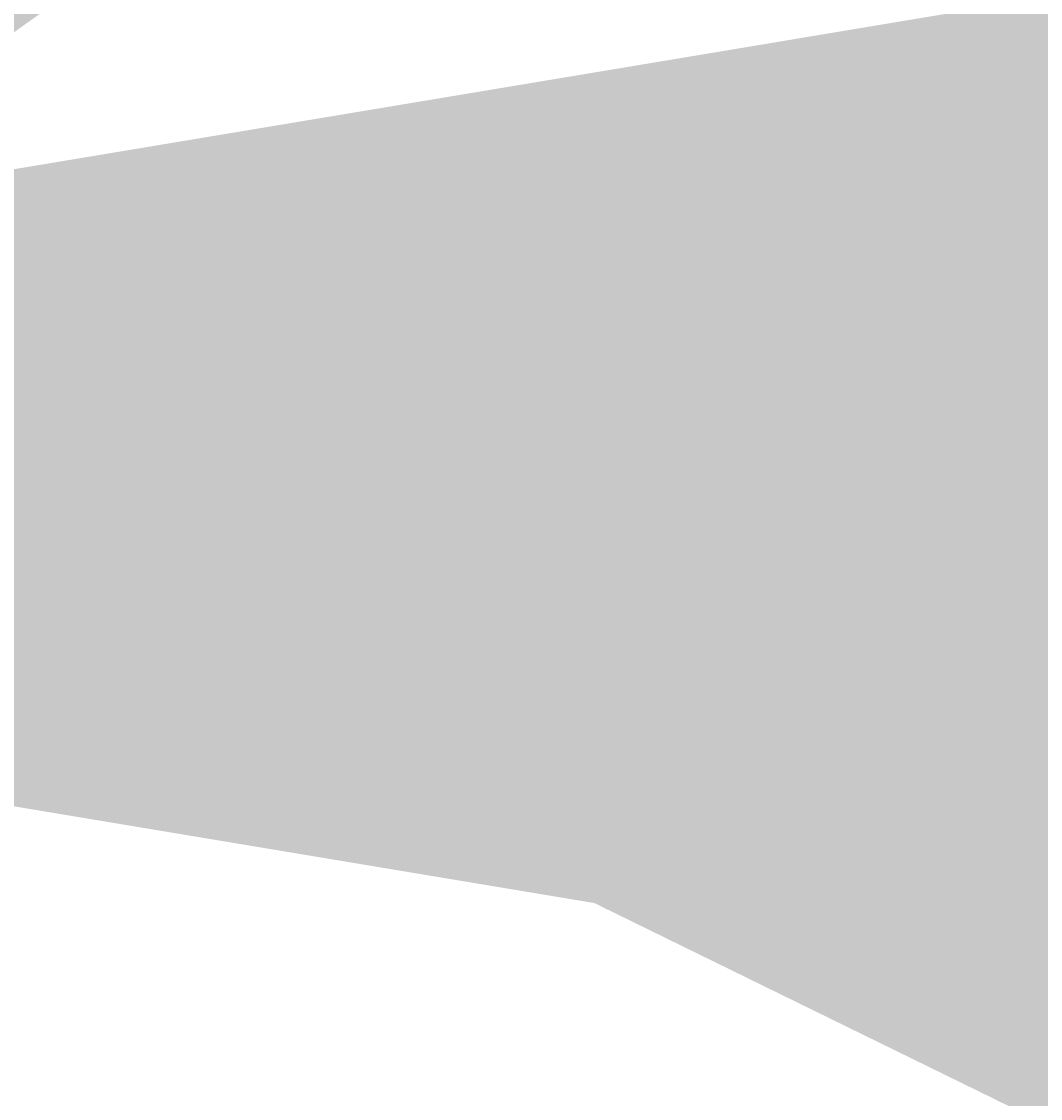
# Model space of a CAD drawing. Units: millimetres. Extents: x -22994 to 29398, y -19990 to 20176.
# Tile 127 of 135: x 480 to 1004, y -212 to 341. Entities that reach past the tile are written whole.
import ezdxf

# ---------------------------------------------------------------- set-up
doc = ezdxf.new("R2010")
doc.units = ezdxf.units.MM
doc.header["$MEASUREMENT"] = 0
doc.layers.add('M-DIMS', color=2, linetype='Continuous', lineweight=18)
doc.styles.get("Standard").update_dxf_attribs({"font": 'arial.ttf'})
doc.dimstyles.get("Standard").update_dxf_attribs({"dimtxt": 0.18, "dimasz": 10000, "dimexe": 0.18, "dimexo": 0.0625, "dimgap": 0.09, "dimtad": 0, "dimtih": 1, "dimtoh": 1, "dimdec": 0, "dimzin": 0, "dimdsep": 46, "dimtxsty": 'Standard', "dimcen": 0.09, "dimadec": 0, "dimazin": 0, "dimtfac": 1, "dimtdec": 0, "dimtofl": 0, "dimtmove": 0, "dimatfit": 3, "dimfxl": 1, "dimtolj": 1, "dimtzin": 0, "dimlwd": 30, "dimarcsym": 0})

# ---------------------------------------------------------------- blocks, each defined once
blk = doc.blocks.new('*D2')
at = {"layer": 'Defpoints', "color": 0, "transparency": 16777216}
for p in [(6.68, 10.27), (290.85, 10.27), (290.85, -5.08)]:
    blk.add_point(p, dxfattribs=at)
at = {"layer": 'M-DIMS', "color": 0, "lineweight": -2, "transparency": 16777216}
for p, q in [((6.68, 10.21), (6.68, -5.26)), ((290.85, 10.21), (290.85, -5.26))]:
    blk.add_line(p, q, dxfattribs=at)
at = {"layer": 'M-DIMS', "color": 0, "lineweight": 30, "transparency": 16777216}
for p, q in [((-9993.32, -5.08), (-19993.32, -5.08)), ((10290.85, -5.08), (20290.85, -5.08))]:
    blk.add_line(p, q, dxfattribs=at)
at = {"layer": 'M-DIMS', "color": 0, "transparency": 16777216}
for points in [[(-9993.32, 1661.59), (-9993.32, -1671.75), (6.68, -5.08)], [(10290.85, 1661.59), (10290.85, -1671.75), (290.85, -5.08)]]:
    blk.add_solid(points, dxfattribs=at)
at = {"layer": 'M-DIMS', "color": 0, "transparency": 16777216, "insert": (148.76, -5.08), "char_height": 0.18, "attachment_point": 5}
blk.add_mtext('\\A1;284.2', dxfattribs=at)
blk = doc.blocks.new('*D3')
at = {"layer": 'Defpoints', "color": 0, "transparency": 16777216}
for p in [(110.26, 204.17), (110.26, 176.37), (95.83, 127.97)]:
    blk.add_point(p, dxfattribs=at)
at = {"layer": 'M-DIMS', "color": 0, "lineweight": 30, "transparency": 16777216}
for p, q in [((-9904.17, 204.17), (-19904.17, 204.17)), ((10110.26, 204.17), (20110.26, 204.17))]:
    blk.add_line(p, q, dxfattribs=at)
at = {"layer": 'M-DIMS', "color": 0, "lineweight": -2, "transparency": 16777216}
for p, q in [((95.83, 128.03), (95.83, 204.35)), ((110.26, 176.43), (110.26, 204.35))]:
    blk.add_line(p, q, dxfattribs=at)
at = {"layer": 'M-DIMS', "color": 0, "transparency": 16777216}
for points in [[(-9904.17, 1870.83), (-9904.17, -1462.5), (95.83, 204.17)], [(10110.26, 1870.83), (10110.26, -1462.5), (110.26, 204.17)]]:
    blk.add_solid(points, dxfattribs=at)
at = {"layer": 'M-DIMS', "color": 0, "transparency": 16777216, "insert": (103.05, 204.17), "char_height": 0.18, "attachment_point": 5}
blk.add_mtext('\\A1;14.432', dxfattribs=at)
blk = doc.blocks.new('*D4')
at = {"layer": 'Defpoints', "color": 0, "transparency": 16777216}
for p in [(116.26, 204.17), (110.26, 176.37), (116.26, 176.37)]:
    blk.add_point(p, dxfattribs=at)
at = {"layer": 'M-DIMS', "color": 0, "lineweight": 30, "transparency": 16777216}
for p, q in [((-9889.74, 204.17), (-19889.74, 204.17)), ((10116.26, 204.17), (20116.26, 204.17))]:
    blk.add_line(p, q, dxfattribs=at)
at = {"layer": 'M-DIMS', "color": 0, "lineweight": -2, "transparency": 16777216}
for p, q in [((110.26, 176.43), (110.26, 204.35)), ((116.26, 176.43), (116.26, 204.35))]:
    blk.add_line(p, q, dxfattribs=at)
at = {"layer": 'M-DIMS', "color": 0, "transparency": 16777216}
for points in [[(-9889.74, 1870.83), (-9889.74, -1462.5), (110.26, 204.17)], [(10116.26, 1870.83), (10116.26, -1462.5), (116.26, 204.17)]]:
    blk.add_solid(points, dxfattribs=at)
at = {"layer": 'M-DIMS', "color": 0, "transparency": 16777216, "insert": (113.26, 204.17), "char_height": 0.18, "attachment_point": 5}
blk.add_mtext('\\A1;6', dxfattribs=at)
blk = doc.blocks.new('*D5')
at = {"layer": 'Defpoints', "color": 0, "transparency": 16777216}
for p in [(181.26, 204.17), (116.26, 176.37), (181.26, 176.37)]:
    blk.add_point(p, dxfattribs=at)
at = {"layer": 'M-DIMS', "color": 0, "lineweight": 30, "transparency": 16777216}
for p, q in [((-9883.74, 204.17), (-19883.74, 204.17)), ((10181.26, 204.17), (20181.26, 204.17))]:
    blk.add_line(p, q, dxfattribs=at)
at = {"layer": 'M-DIMS', "color": 0, "lineweight": -2, "transparency": 16777216}
for p, q in [((116.26, 176.43), (116.26, 204.35)), ((181.26, 176.43), (181.26, 204.35))]:
    blk.add_line(p, q, dxfattribs=at)
at = {"layer": 'M-DIMS', "color": 0, "transparency": 16777216}
for points in [[(-9883.74, 1870.83), (-9883.74, -1462.5), (116.26, 204.17)], [(10181.26, 1870.83), (10181.26, -1462.5), (181.26, 204.17)]]:
    blk.add_solid(points, dxfattribs=at)
at = {"layer": 'M-DIMS', "color": 0, "transparency": 16777216, "insert": (148.76, 204.17), "char_height": 0.18, "attachment_point": 5}
blk.add_mtext('\\A1;65', dxfattribs=at)
blk = doc.blocks.new('*D6')
at = {"layer": 'Defpoints', "color": 0, "transparency": 16777216}
for p in [(187.26, 204.17), (181.26, 176.37), (187.26, 176.37)]:
    blk.add_point(p, dxfattribs=at)
at = {"layer": 'M-DIMS', "color": 0, "lineweight": 30, "transparency": 16777216}
for p, q in [((-9818.74, 204.17), (-19818.74, 204.17)), ((10187.26, 204.17), (20187.26, 204.17))]:
    blk.add_line(p, q, dxfattribs=at)
at = {"layer": 'M-DIMS', "color": 0, "lineweight": -2, "transparency": 16777216}
for p, q in [((181.26, 176.43), (181.26, 204.35)), ((187.26, 176.43), (187.26, 204.35))]:
    blk.add_line(p, q, dxfattribs=at)
at = {"layer": 'M-DIMS', "color": 0, "transparency": 16777216}
for points in [[(-9818.74, 1870.83), (-9818.74, -1462.5), (181.26, 204.17)], [(10187.26, 1870.83), (10187.26, -1462.5), (187.26, 204.17)]]:
    blk.add_solid(points, dxfattribs=at)
at = {"layer": 'M-DIMS', "color": 0, "transparency": 16777216, "insert": (184.26, 204.17), "char_height": 0.18, "attachment_point": 5}
blk.add_mtext('\\A1;6', dxfattribs=at)
blk = doc.blocks.new('*D7')
at = {"layer": 'Defpoints', "color": 0, "transparency": 16777216}
for p in [(201.7, 204.17), (187.26, 176.37), (201.7, 127.97)]:
    blk.add_point(p, dxfattribs=at)
at = {"layer": 'M-DIMS', "color": 0, "lineweight": 30, "transparency": 16777216}
for p, q in [((-9812.74, 204.17), (-19812.74, 204.17)), ((10201.7, 204.17), (20201.7, 204.17))]:
    blk.add_line(p, q, dxfattribs=at)
at = {"layer": 'M-DIMS', "color": 0, "lineweight": -2, "transparency": 16777216}
for p, q in [((187.26, 176.43), (187.26, 204.35)), ((201.7, 128.03), (201.7, 204.35))]:
    blk.add_line(p, q, dxfattribs=at)
at = {"layer": 'M-DIMS', "color": 0, "transparency": 16777216}
for points in [[(-9812.74, 1870.83), (-9812.74, -1462.5), (187.26, 204.17)], [(10201.7, 1870.83), (10201.7, -1462.5), (201.7, 204.17)]]:
    blk.add_solid(points, dxfattribs=at)
at = {"layer": 'M-DIMS', "color": 0, "transparency": 16777216, "insert": (194.48, 204.17), "char_height": 0.18, "attachment_point": 5}
blk.add_mtext('\\A1;14.432', dxfattribs=at)
blk = doc.blocks.new('*D8')
at = {"layer": 'Defpoints', "color": 0, "transparency": 16777216}
for p in [(227.65, 204.17), (227.65, 146.73), (201.7, 127.97)]:
    blk.add_point(p, dxfattribs=at)
at = {"layer": 'M-DIMS', "color": 0, "lineweight": 30, "transparency": 16777216}
for p, q in [((-9798.3, 204.17), (-19798.3, 204.17)), ((10227.65, 204.17), (20227.65, 204.17))]:
    blk.add_line(p, q, dxfattribs=at)
at = {"layer": 'M-DIMS', "color": 0, "lineweight": -2, "transparency": 16777216}
for p, q in [((201.7, 128.03), (201.7, 204.35)), ((227.65, 146.79), (227.65, 204.35))]:
    blk.add_line(p, q, dxfattribs=at)
at = {"layer": 'M-DIMS', "color": 0, "transparency": 16777216}
for points in [[(-9798.3, 1870.83), (-9798.3, -1462.5), (201.7, 204.17)], [(10227.65, 1870.83), (10227.65, -1462.5), (227.65, 204.17)]]:
    blk.add_solid(points, dxfattribs=at)
at = {"layer": 'M-DIMS', "color": 0, "transparency": 16777216, "insert": (214.67, 204.17), "char_height": 0.18, "attachment_point": 5}
blk.add_mtext('\\A1;25.95', dxfattribs=at)
blk = doc.blocks.new('*D9')
at = {"layer": 'Defpoints', "color": 0, "transparency": 16777216}
for p in [(187.26, 176.37), (306.2, 176.37), (290.85, 10.27)]:
    blk.add_point(p, dxfattribs=at)
at = {"layer": 'M-DIMS', "color": 0, "lineweight": 30, "transparency": 16777216}
for p, q in [((306.2, 10176.37), (306.2, 20176.37)), ((306.2, -9989.73), (306.2, -19989.73))]:
    blk.add_line(p, q, dxfattribs=at)
at = {"layer": 'M-DIMS', "color": 0, "lineweight": -2, "transparency": 16777216}
for p, q in [((187.33, 176.37), (306.38, 176.37)), ((290.91, 10.27), (306.38, 10.27))]:
    blk.add_line(p, q, dxfattribs=at)
at = {"layer": 'M-DIMS', "color": 0, "transparency": 16777216}
for points in [[(-1360.46, 10176.37), (1972.87, 10176.37), (306.2, 176.37)], [(-1360.46, -9989.73), (1972.87, -9989.73), (306.2, 10.27)]]:
    blk.add_solid(points, dxfattribs=at)
at = {"layer": 'M-DIMS', "color": 0, "transparency": 16777216, "insert": (306.2, 93.32), "char_height": 0.18, "attachment_point": 5}
blk.add_mtext('\\A1;166.1', dxfattribs=at)
blk = doc.blocks.new('*D10')
at = {"layer": 'Defpoints', "color": 0, "transparency": 16777216}
for p in [(125.65, 136.07), (133.35, 136.07), (133.35, -5.08)]:
    blk.add_point(p, dxfattribs=at)
at = {"layer": 'M-DIMS', "color": 0, "lineweight": -2, "transparency": 16777216}
for p, q in [((125.65, 136.01), (125.65, -5.26)), ((133.35, 136.01), (133.35, -5.26))]:
    blk.add_line(p, q, dxfattribs=at)
at = {"layer": 'M-DIMS', "color": 0, "lineweight": 30, "transparency": 16777216}
for p, q in [((-9874.35, -5.08), (-19874.35, -5.08)), ((10133.35, -5.08), (20133.35, -5.08))]:
    blk.add_line(p, q, dxfattribs=at)
at = {"layer": 'M-DIMS', "color": 0, "transparency": 16777216}
for points in [[(-9874.35, 1661.59), (-9874.35, -1671.75), (125.65, -5.08)], [(10133.35, 1661.59), (10133.35, -1671.75), (133.35, -5.08)]]:
    blk.add_solid(points, dxfattribs=at)
at = {"layer": 'M-DIMS', "color": 0, "transparency": 16777216, "insert": (129.5, -5.08), "char_height": 0.18, "attachment_point": 5}
blk.add_mtext('\\A1;7.696', dxfattribs=at)
blk = doc.blocks.new('*D11')
at = {"layer": 'Defpoints', "color": 0, "transparency": 16777216}
for p in [(133.35, 136.07), (135.65, 136.07), (135.65, -5.08)]:
    blk.add_point(p, dxfattribs=at)
at = {"layer": 'M-DIMS', "color": 0, "lineweight": -2, "transparency": 16777216}
for p, q in [((133.35, 136.01), (133.35, -5.26)), ((135.65, 136.01), (135.65, -5.26))]:
    blk.add_line(p, q, dxfattribs=at)
at = {"layer": 'M-DIMS', "color": 0, "lineweight": 30, "transparency": 16777216}
for p, q in [((-9866.65, -5.08), (-19866.65, -5.08)), ((10135.65, -5.08), (20135.65, -5.08))]:
    blk.add_line(p, q, dxfattribs=at)
at = {"layer": 'M-DIMS', "color": 0, "transparency": 16777216}
for points in [[(-9866.65, 1661.59), (-9866.65, -1671.75), (133.35, -5.08)], [(10135.65, 1661.59), (10135.65, -1671.75), (135.65, -5.08)]]:
    blk.add_solid(points, dxfattribs=at)
at = {"layer": 'M-DIMS', "color": 0, "transparency": 16777216, "insert": (134.5, -5.08), "char_height": 0.18, "attachment_point": 5}
blk.add_mtext('\\A1;2.304', dxfattribs=at)
blk = doc.blocks.new('*D12')
at = {"layer": 'Defpoints', "color": 0, "transparency": 16777216}
for p in [(135.65, 136.07), (145.65, 136.07), (145.65, -5.08)]:
    blk.add_point(p, dxfattribs=at)
at = {"layer": 'M-DIMS', "color": 0, "lineweight": -2, "transparency": 16777216}
for p, q in [((135.65, 136.01), (135.65, -5.26)), ((145.65, 136.01), (145.65, -5.26))]:
    blk.add_line(p, q, dxfattribs=at)
at = {"layer": 'M-DIMS', "color": 0, "lineweight": 30, "transparency": 16777216}
for p, q in [((-9864.35, -5.08), (-19864.35, -5.08)), ((10145.65, -5.08), (20145.65, -5.08))]:
    blk.add_line(p, q, dxfattribs=at)
at = {"layer": 'M-DIMS', "color": 0, "transparency": 16777216}
for points in [[(-9864.35, 1661.59), (-9864.35, -1671.75), (135.65, -5.08)], [(10145.65, 1661.59), (10145.65, -1671.75), (145.65, -5.08)]]:
    blk.add_solid(points, dxfattribs=at)
at = {"layer": 'M-DIMS', "color": 0, "transparency": 16777216, "insert": (140.65, -5.08), "char_height": 0.18, "attachment_point": 5}
blk.add_mtext('\\A1;10', dxfattribs=at)
blk = doc.blocks.new('*D13')
at = {"layer": 'Defpoints', "color": 0, "transparency": 16777216}
for p in [(145.65, 136.07), (155.65, 136.07), (155.65, -5.08)]:
    blk.add_point(p, dxfattribs=at)
at = {"layer": 'M-DIMS', "color": 0, "lineweight": -2, "transparency": 16777216}
for p, q in [((145.65, 136.01), (145.65, -5.26)), ((155.65, 136.01), (155.65, -5.26))]:
    blk.add_line(p, q, dxfattribs=at)
at = {"layer": 'M-DIMS', "color": 0, "lineweight": 30, "transparency": 16777216}
for p, q in [((-9854.35, -5.08), (-19854.35, -5.08)), ((10155.65, -5.08), (20155.65, -5.08))]:
    blk.add_line(p, q, dxfattribs=at)
at = {"layer": 'M-DIMS', "color": 0, "transparency": 16777216}
for points in [[(-9854.35, 1661.59), (-9854.35, -1671.75), (145.65, -5.08)], [(10155.65, 1661.59), (10155.65, -1671.75), (155.65, -5.08)]]:
    blk.add_solid(points, dxfattribs=at)
at = {"layer": 'M-DIMS', "color": 0, "transparency": 16777216, "insert": (150.65, -5.08), "char_height": 0.18, "attachment_point": 5}
blk.add_mtext('\\A1;10', dxfattribs=at)
blk = doc.blocks.new('*D14')
at = {"layer": 'Defpoints', "color": 0, "transparency": 16777216}
for p in [(155.65, 136.07), (165.65, 136.07), (165.65, -5.08)]:
    blk.add_point(p, dxfattribs=at)
at = {"layer": 'M-DIMS', "color": 0, "lineweight": -2, "transparency": 16777216}
for p, q in [((155.65, 136.01), (155.65, -5.26)), ((165.65, 136.01), (165.65, -5.26))]:
    blk.add_line(p, q, dxfattribs=at)
at = {"layer": 'M-DIMS', "color": 0, "lineweight": 30, "transparency": 16777216}
for p, q in [((-9844.35, -5.08), (-19844.35, -5.08)), ((10165.65, -5.08), (20165.65, -5.08))]:
    blk.add_line(p, q, dxfattribs=at)
at = {"layer": 'M-DIMS', "color": 0, "transparency": 16777216}
for points in [[(-9844.35, 1661.59), (-9844.35, -1671.75), (155.65, -5.08)], [(10165.65, 1661.59), (10165.65, -1671.75), (165.65, -5.08)]]:
    blk.add_solid(points, dxfattribs=at)
at = {"layer": 'M-DIMS', "color": 0, "transparency": 16777216, "insert": (160.65, -5.08), "char_height": 0.18, "attachment_point": 5}
blk.add_mtext('\\A1;10', dxfattribs=at)
blk = doc.blocks.new('*D15')
at = {"layer": 'Defpoints', "color": 0, "transparency": 16777216}
for p in [(173.35, 154.79), (173.35, 136.07), (306.2, 136.07)]:
    blk.add_point(p, dxfattribs=at)
at = {"layer": 'M-DIMS', "color": 0, "lineweight": 30, "transparency": 16777216}
for p, q in [((306.2, 10154.79), (306.2, 20154.79)), ((306.2, -9863.93), (306.2, -19863.93))]:
    blk.add_line(p, q, dxfattribs=at)
at = {"layer": 'M-DIMS', "color": 0, "lineweight": -2, "transparency": 16777216}
for p, q in [((173.41, 154.79), (306.38, 154.79)), ((173.41, 136.07), (306.38, 136.07))]:
    blk.add_line(p, q, dxfattribs=at)
at = {"layer": 'M-DIMS', "color": 0, "transparency": 16777216}
for points in [[(-1360.46, 10154.79), (1972.87, 10154.79), (306.2, 154.79)], [(-1360.46, -9863.93), (1972.87, -9863.93), (306.2, 136.07)]]:
    blk.add_solid(points, dxfattribs=at)
at = {"layer": 'M-DIMS', "color": 0, "transparency": 16777216, "insert": (306.2, 145.43), "char_height": 0.18, "attachment_point": 5}
blk.add_mtext('\\A1;18.717', dxfattribs=at)
blk = doc.blocks.new('*D16')
at = {"layer": 'Defpoints', "color": 0, "transparency": 16777216}
for p in [(120.17, 204.17), (110.47, 48.03), (120.17, 48.03)]:
    blk.add_point(p, dxfattribs=at)
at = {"layer": 'M-DIMS', "color": 0, "lineweight": 30, "transparency": 16777216}
for p, q in [((-9889.53, 204.17), (-19889.53, 204.17)), ((10120.17, 204.17), (20120.17, 204.17))]:
    blk.add_line(p, q, dxfattribs=at)
at = {"layer": 'M-DIMS', "color": 0, "lineweight": -2, "transparency": 16777216}
for p, q in [((110.47, 48.1), (110.47, 204.35)), ((120.17, 48.1), (120.17, 204.35))]:
    blk.add_line(p, q, dxfattribs=at)
at = {"layer": 'M-DIMS', "color": 0, "transparency": 16777216}
for points in [[(-9889.53, 1870.83), (-9889.53, -1462.5), (110.47, 204.17)], [(10120.17, 1870.83), (10120.17, -1462.5), (120.17, 204.17)]]:
    blk.add_solid(points, dxfattribs=at)
at = {"layer": 'M-DIMS', "color": 0, "transparency": 16777216, "insert": (115.32, 204.17), "char_height": 0.18, "attachment_point": 5}
blk.add_mtext('\\A1;9.704', dxfattribs=at)
blk = doc.blocks.new('*D17')
at = {"layer": 'Defpoints', "color": 0, "transparency": 16777216}
for p in [(126.17, 204.17), (120.17, 48.03), (126.17, 48.03)]:
    blk.add_point(p, dxfattribs=at)
at = {"layer": 'M-DIMS', "color": 0, "lineweight": 30, "transparency": 16777216}
for p, q in [((-9879.83, 204.17), (-19879.83, 204.17)), ((10126.17, 204.17), (20126.17, 204.17))]:
    blk.add_line(p, q, dxfattribs=at)
at = {"layer": 'M-DIMS', "color": 0, "lineweight": -2, "transparency": 16777216}
for p, q in [((120.17, 48.1), (120.17, 204.35)), ((126.17, 48.1), (126.17, 204.35))]:
    blk.add_line(p, q, dxfattribs=at)
at = {"layer": 'M-DIMS', "color": 0, "transparency": 16777216}
for points in [[(-9879.83, 1870.83), (-9879.83, -1462.5), (120.17, 204.17)], [(10126.17, 1870.83), (10126.17, -1462.5), (126.17, 204.17)]]:
    blk.add_solid(points, dxfattribs=at)
at = {"layer": 'M-DIMS', "color": 0, "transparency": 16777216, "insert": (123.17, 204.17), "char_height": 0.18, "attachment_point": 5}
blk.add_mtext('\\A1;6', dxfattribs=at)
blk = doc.blocks.new('*D18')
at = {"layer": 'Defpoints', "color": 0, "transparency": 16777216}
for p in [(132.17, 204.17), (126.17, 48.03), (132.17, 48.03)]:
    blk.add_point(p, dxfattribs=at)
at = {"layer": 'M-DIMS', "color": 0, "lineweight": 30, "transparency": 16777216}
for p, q in [((-9873.83, 204.17), (-19873.83, 204.17)), ((10132.17, 204.17), (20132.17, 204.17))]:
    blk.add_line(p, q, dxfattribs=at)
at = {"layer": 'M-DIMS', "color": 0, "lineweight": -2, "transparency": 16777216}
for p, q in [((126.17, 48.1), (126.17, 204.35)), ((132.17, 48.1), (132.17, 204.35))]:
    blk.add_line(p, q, dxfattribs=at)
at = {"layer": 'M-DIMS', "color": 0, "transparency": 16777216}
for points in [[(-9873.83, 1870.83), (-9873.83, -1462.5), (126.17, 204.17)], [(10132.17, 1870.83), (10132.17, -1462.5), (132.17, 204.17)]]:
    blk.add_solid(points, dxfattribs=at)
at = {"layer": 'M-DIMS', "color": 0, "transparency": 16777216, "insert": (129.17, 204.17), "char_height": 0.18, "attachment_point": 5}
blk.add_mtext('\\A1;6', dxfattribs=at)
blk = doc.blocks.new('*D19')
at = {"layer": 'Defpoints', "color": 0, "transparency": 16777216}
for p in [(138.17, 204.17), (132.17, 48.03), (138.17, 48.03)]:
    blk.add_point(p, dxfattribs=at)
at = {"layer": 'M-DIMS', "color": 0, "lineweight": 30, "transparency": 16777216}
for p, q in [((-9867.83, 204.17), (-19867.83, 204.17)), ((10138.17, 204.17), (20138.17, 204.17))]:
    blk.add_line(p, q, dxfattribs=at)
at = {"layer": 'M-DIMS', "color": 0, "lineweight": -2, "transparency": 16777216}
for p, q in [((132.17, 48.1), (132.17, 204.35)), ((138.17, 48.1), (138.17, 204.35))]:
    blk.add_line(p, q, dxfattribs=at)
at = {"layer": 'M-DIMS', "color": 0, "transparency": 16777216}
for points in [[(-9867.83, 1870.83), (-9867.83, -1462.5), (132.17, 204.17)], [(10138.17, 1870.83), (10138.17, -1462.5), (138.17, 204.17)]]:
    blk.add_solid(points, dxfattribs=at)
at = {"layer": 'M-DIMS', "color": 0, "transparency": 16777216, "insert": (135.17, 204.17), "char_height": 0.18, "attachment_point": 5}
blk.add_mtext('\\A1;6', dxfattribs=at)
blk = doc.blocks.new('*D20')
at = {"layer": 'Defpoints', "color": 0, "transparency": 16777216}
for p in [(144.17, 204.17), (138.17, 48.03), (144.17, 48.03)]:
    blk.add_point(p, dxfattribs=at)
at = {"layer": 'M-DIMS', "color": 0, "lineweight": 30, "transparency": 16777216}
for p, q in [((-9861.83, 204.17), (-19861.83, 204.17)), ((10144.17, 204.17), (20144.17, 204.17))]:
    blk.add_line(p, q, dxfattribs=at)
at = {"layer": 'M-DIMS', "color": 0, "lineweight": -2, "transparency": 16777216}
for p, q in [((138.17, 48.1), (138.17, 204.35)), ((144.17, 48.1), (144.17, 204.35))]:
    blk.add_line(p, q, dxfattribs=at)
at = {"layer": 'M-DIMS', "color": 0, "transparency": 16777216}
for points in [[(-9861.83, 1870.83), (-9861.83, -1462.5), (138.17, 204.17)], [(10144.17, 1870.83), (10144.17, -1462.5), (144.17, 204.17)]]:
    blk.add_solid(points, dxfattribs=at)
at = {"layer": 'M-DIMS', "color": 0, "transparency": 16777216, "insert": (141.17, 204.17), "char_height": 0.18, "attachment_point": 5}
blk.add_mtext('\\A1;6', dxfattribs=at)
blk = doc.blocks.new('*D21')
at = {"layer": 'Defpoints', "color": 0, "transparency": 16777216}
for p in [(149.12, 204.17), (144.17, 48.03), (149.12, 48.03)]:
    blk.add_point(p, dxfattribs=at)
at = {"layer": 'M-DIMS', "color": 0, "lineweight": 30, "transparency": 16777216}
for p, q in [((-9855.83, 204.17), (-19855.83, 204.17)), ((10149.12, 204.17), (20149.12, 204.17))]:
    blk.add_line(p, q, dxfattribs=at)
at = {"layer": 'M-DIMS', "color": 0, "lineweight": -2, "transparency": 16777216}
for p, q in [((144.17, 48.1), (144.17, 204.35)), ((149.12, 48.1), (149.12, 204.35))]:
    blk.add_line(p, q, dxfattribs=at)
at = {"layer": 'M-DIMS', "color": 0, "transparency": 16777216}
for points in [[(-9855.83, 1870.83), (-9855.83, -1462.5), (144.17, 204.17)], [(10149.12, 1870.83), (10149.12, -1462.5), (149.12, 204.17)]]:
    blk.add_solid(points, dxfattribs=at)
at = {"layer": 'M-DIMS', "color": 0, "transparency": 16777216, "insert": (146.64, 204.17), "char_height": 0.18, "attachment_point": 5}
blk.add_mtext('\\A1;4.945', dxfattribs=at)
blk = doc.blocks.new('*D22')
at = {"layer": 'Defpoints', "color": 0, "transparency": 16777216}
for p in [(149.12, 30.99), (155.12, 30.99), (155.12, -5.08)]:
    blk.add_point(p, dxfattribs=at)
at = {"layer": 'M-DIMS', "color": 0, "lineweight": -2, "transparency": 16777216}
for p, q in [((149.12, 30.93), (149.12, -5.26)), ((155.12, 30.93), (155.12, -5.26))]:
    blk.add_line(p, q, dxfattribs=at)
at = {"layer": 'M-DIMS', "color": 0, "lineweight": 30, "transparency": 16777216}
for p, q in [((-9850.88, -5.08), (-19850.88, -5.08)), ((10155.12, -5.08), (20155.12, -5.08))]:
    blk.add_line(p, q, dxfattribs=at)
at = {"layer": 'M-DIMS', "color": 0, "transparency": 16777216}
for points in [[(-9850.88, 1661.59), (-9850.88, -1671.75), (149.12, -5.08)], [(10155.12, 1661.59), (10155.12, -1671.75), (155.12, -5.08)]]:
    blk.add_solid(points, dxfattribs=at)
at = {"layer": 'M-DIMS', "color": 0, "transparency": 16777216, "insert": (152.12, -5.08), "char_height": 0.18, "attachment_point": 5}
blk.add_mtext('\\A1;6', dxfattribs=at)
blk = doc.blocks.new('*D23')
at = {"layer": 'Defpoints', "color": 0, "transparency": 16777216}
for p in [(155.12, 30.99), (161.12, 30.99), (161.12, -5.08)]:
    blk.add_point(p, dxfattribs=at)
at = {"layer": 'M-DIMS', "color": 0, "lineweight": -2, "transparency": 16777216}
for p, q in [((155.12, 30.93), (155.12, -5.26)), ((161.12, 30.93), (161.12, -5.26))]:
    blk.add_line(p, q, dxfattribs=at)
at = {"layer": 'M-DIMS', "color": 0, "lineweight": 30, "transparency": 16777216}
for p, q in [((-9844.88, -5.08), (-19844.88, -5.08)), ((10161.12, -5.08), (20161.12, -5.08))]:
    blk.add_line(p, q, dxfattribs=at)
at = {"layer": 'M-DIMS', "color": 0, "transparency": 16777216}
for points in [[(-9844.88, 1661.59), (-9844.88, -1671.75), (155.12, -5.08)], [(10161.12, 1661.59), (10161.12, -1671.75), (161.12, -5.08)]]:
    blk.add_solid(points, dxfattribs=at)
at = {"layer": 'M-DIMS', "color": 0, "transparency": 16777216, "insert": (158.12, -5.08), "char_height": 0.18, "attachment_point": 5}
blk.add_mtext('\\A1;6', dxfattribs=at)
blk = doc.blocks.new('*D24')
at = {"layer": 'Defpoints', "color": 0, "transparency": 16777216}
for p in [(161.12, 30.99), (166.44, 30.99), (166.44, -5.08)]:
    blk.add_point(p, dxfattribs=at)
at = {"layer": 'M-DIMS', "color": 0, "lineweight": -2, "transparency": 16777216}
for p, q in [((161.12, 30.93), (161.12, -5.26)), ((166.44, 30.93), (166.44, -5.26))]:
    blk.add_line(p, q, dxfattribs=at)
at = {"layer": 'M-DIMS', "color": 0, "lineweight": 30, "transparency": 16777216}
for p, q in [((-9838.88, -5.08), (-19838.88, -5.08)), ((10166.44, -5.08), (20166.44, -5.08))]:
    blk.add_line(p, q, dxfattribs=at)
at = {"layer": 'M-DIMS', "color": 0, "transparency": 16777216}
for points in [[(-9838.88, 1661.59), (-9838.88, -1671.75), (161.12, -5.08)], [(10166.44, 1661.59), (10166.44, -1671.75), (166.44, -5.08)]]:
    blk.add_solid(points, dxfattribs=at)
at = {"layer": 'M-DIMS', "color": 0, "transparency": 16777216, "insert": (163.78, -5.08), "char_height": 0.18, "attachment_point": 5}
blk.add_mtext('\\A1;5.323', dxfattribs=at)
blk = doc.blocks.new('*D25')
at = {"layer": 'Defpoints', "color": 0, "transparency": 16777216}
for p in [(166.44, 30.99), (172.44, 30.99), (172.44, -5.08)]:
    blk.add_point(p, dxfattribs=at)
at = {"layer": 'M-DIMS', "color": 0, "lineweight": -2, "transparency": 16777216}
for p, q in [((166.44, 30.93), (166.44, -5.26)), ((172.44, 30.93), (172.44, -5.26))]:
    blk.add_line(p, q, dxfattribs=at)
at = {"layer": 'M-DIMS', "color": 0, "lineweight": 30, "transparency": 16777216}
for p, q in [((-9833.56, -5.08), (-19833.56, -5.08)), ((10172.44, -5.08), (20172.44, -5.08))]:
    blk.add_line(p, q, dxfattribs=at)
at = {"layer": 'M-DIMS', "color": 0, "transparency": 16777216}
for points in [[(-9833.56, 1661.59), (-9833.56, -1671.75), (166.44, -5.08)], [(10172.44, 1661.59), (10172.44, -1671.75), (172.44, -5.08)]]:
    blk.add_solid(points, dxfattribs=at)
at = {"layer": 'M-DIMS', "color": 0, "transparency": 16777216, "insert": (169.44, -5.08), "char_height": 0.18, "attachment_point": 5}
blk.add_mtext('\\A1;6', dxfattribs=at)
blk = doc.blocks.new('*D26')
at = {"layer": 'Defpoints', "color": 0, "transparency": 16777216}
for p in [(172.44, 30.99), (178.44, 30.99), (178.44, -5.08)]:
    blk.add_point(p, dxfattribs=at)
at = {"layer": 'M-DIMS', "color": 0, "lineweight": -2, "transparency": 16777216}
for p, q in [((172.44, 30.93), (172.44, -5.26)), ((178.44, 30.93), (178.44, -5.26))]:
    blk.add_line(p, q, dxfattribs=at)
at = {"layer": 'M-DIMS', "color": 0, "lineweight": 30, "transparency": 16777216}
for p, q in [((-9827.56, -5.08), (-19827.56, -5.08)), ((10178.44, -5.08), (20178.44, -5.08))]:
    blk.add_line(p, q, dxfattribs=at)
at = {"layer": 'M-DIMS', "color": 0, "transparency": 16777216}
for points in [[(-9827.56, 1661.59), (-9827.56, -1671.75), (172.44, -5.08)], [(10178.44, 1661.59), (10178.44, -1671.75), (178.44, -5.08)]]:
    blk.add_solid(points, dxfattribs=at)
at = {"layer": 'M-DIMS', "color": 0, "transparency": 16777216, "insert": (175.44, -5.08), "char_height": 0.18, "attachment_point": 5}
blk.add_mtext('\\A1;6', dxfattribs=at)
blk = doc.blocks.new('*D27')
at = {"layer": 'Defpoints', "color": 0, "transparency": 16777216}
for p in [(178.44, 30.99), (188.12, 30.99), (188.12, -5.08)]:
    blk.add_point(p, dxfattribs=at)
at = {"layer": 'M-DIMS', "color": 0, "lineweight": -2, "transparency": 16777216}
for p, q in [((178.44, 30.93), (178.44, -5.26)), ((188.12, 30.93), (188.12, -5.26))]:
    blk.add_line(p, q, dxfattribs=at)
at = {"layer": 'M-DIMS', "color": 0, "lineweight": 30, "transparency": 16777216}
for p, q in [((-9821.56, -5.08), (-19821.56, -5.08)), ((10188.12, -5.08), (20188.12, -5.08))]:
    blk.add_line(p, q, dxfattribs=at)
at = {"layer": 'M-DIMS', "color": 0, "transparency": 16777216}
for points in [[(-9821.56, 1661.59), (-9821.56, -1671.75), (178.44, -5.08)], [(10188.12, 1661.59), (10188.12, -1671.75), (188.12, -5.08)]]:
    blk.add_solid(points, dxfattribs=at)
at = {"layer": 'M-DIMS', "color": 0, "transparency": 16777216, "insert": (183.28, -5.08), "char_height": 0.18, "attachment_point": 5}
blk.add_mtext('\\A1;9.679', dxfattribs=at)
blk = doc.blocks.new('*D28')
at = {"layer": 'Defpoints', "color": 0, "transparency": 16777216}
for p in [(188.12, 48.03), (306.2, 48.03), (188.12, 30.99)]:
    blk.add_point(p, dxfattribs=at)
at = {"layer": 'M-DIMS', "color": 0, "lineweight": 30, "transparency": 16777216}
for p, q in [((306.2, 10048.03), (306.2, 20048.03)), ((306.2, -9969.01), (306.2, -19969.01))]:
    blk.add_line(p, q, dxfattribs=at)
at = {"layer": 'M-DIMS', "color": 0, "lineweight": -2, "transparency": 16777216}
for p, q in [((188.18, 48.03), (306.38, 48.03)), ((188.18, 30.99), (306.38, 30.99))]:
    blk.add_line(p, q, dxfattribs=at)
at = {"layer": 'M-DIMS', "color": 0, "transparency": 16777216}
for points in [[(-1360.46, 10048.03), (1972.87, 10048.03), (306.2, 48.03)], [(-1360.46, -9969.01), (1972.87, -9969.01), (306.2, 30.99)]]:
    blk.add_solid(points, dxfattribs=at)
at = {"layer": 'M-DIMS', "color": 0, "transparency": 16777216, "insert": (306.2, 39.51), "char_height": 0.18, "attachment_point": 5}
blk.add_mtext('\\A1;17.045', dxfattribs=at)
blk = doc.blocks.new('*D29')
at = {"layer": 'Defpoints', "color": 0, "transparency": 16777216}
for p in [(36.8, 80.04), (64.03, 80.04)]:
    blk.add_point(p, dxfattribs=at)
at = {"layer": 'M-DIMS', "color": 0, "lineweight": -2, "transparency": 16777216}
for p, q in [((50.33, 80.04), (50.51, 80.04)), ((50.42, 79.96), (50.42, 80.14))]:
    blk.add_line(p, q, dxfattribs=at)
at = {"layer": 'M-DIMS', "color": 0, "lineweight": 30, "transparency": 16777216}
blk.add_line((20064.03, 80.03), (10064.03, 80.04), dxfattribs=at)
at = {"layer": 'M-DIMS', "color": 0, "transparency": 16777216}
blk.add_solid([(10064.03, 1746.7), (10064.03, -1586.63), (64.03, 80.04)], dxfattribs=at)
at = {"layer": 'M-DIMS', "color": 0, "transparency": 16777216, "insert": (20064.52, 80.03), "char_height": 0.18, "attachment_point": 5}
blk.add_mtext('\\A1;∅27.23', dxfattribs=at)
blk = doc.blocks.new('*D30')
at = {"layer": 'Defpoints', "color": 0, "transparency": 16777216}
for p in [(216.31, 146.73), (238.98, 146.73)]:
    blk.add_point(p, dxfattribs=at)
at = {"layer": 'M-DIMS', "color": 0, "lineweight": -2, "transparency": 16777216}
for p, q in [((227.56, 146.73), (227.74, 146.73)), ((227.65, 146.64), (227.65, 146.82))]:
    blk.add_line(p, q, dxfattribs=at)
at = {"layer": 'M-DIMS', "color": 0, "lineweight": 30, "transparency": 16777216}
blk.add_line((20238.98, 147.5), (10238.98, 147.11), dxfattribs=at)
at = {"layer": 'M-DIMS', "color": 0, "transparency": 16777216}
blk.add_solid([(10238.92, 1813.78), (10239.05, -1519.55), (238.98, 146.73)], dxfattribs=at)
at = {"layer": 'M-DIMS', "color": 0, "transparency": 16777216, "insert": (20239.54, 147.5), "char_height": 0.18, "attachment_point": 5}
blk.add_mtext('\\A1;∅22.667', dxfattribs=at)
blk = doc.blocks.new('*D31')
at = {"layer": 'Defpoints', "color": 0, "transparency": 16777216}
for p in [(223.16, 146.73), (232.13, 146.73)]:
    blk.add_point(p, dxfattribs=at)
at = {"layer": 'M-DIMS', "color": 0, "lineweight": -2, "transparency": 16777216}
for p, q in [((227.56, 146.73), (227.74, 146.73)), ((227.65, 146.64), (227.65, 146.82))]:
    blk.add_line(p, q, dxfattribs=at)
at = {"layer": 'M-DIMS', "color": 0, "lineweight": 30, "transparency": 16777216}
blk.add_line((20232.13, 148.67), (10232.13, 147.7), dxfattribs=at)
at = {"layer": 'M-DIMS', "color": 0, "transparency": 16777216}
blk.add_solid([(10231.97, 1814.36), (10232.29, -1518.97), (232.13, 146.73)], dxfattribs=at)
at = {"layer": 'M-DIMS', "color": 0, "transparency": 16777216, "insert": (20232.62, 148.67), "char_height": 0.18, "attachment_point": 5}
blk.add_mtext('\\A1;∅8.969', dxfattribs=at)
blk = doc.blocks.new('*D33')
at = {"layer": 'Defpoints', "color": 0, "transparency": 16777216}
for p in [(229.56, 154.38), (233, 153.35)]:
    blk.add_point(p, dxfattribs=at)
at = {"layer": 'M-DIMS', "color": 0, "lineweight": -2, "transparency": 16777216}
for p, q in [((229.47, 154.38), (229.65, 154.38)), ((229.56, 154.29), (229.56, 154.47))]:
    blk.add_line(p, q, dxfattribs=at)
at = {"layer": 'M-DIMS', "color": 0, "lineweight": 30, "transparency": 16777216}
for p, q in [((19396.34, -5570.84), (9814.67, -2708.74)), ((29396.34, -5570.84), (19396.34, -5570.84))]:
    blk.add_line(p, q, dxfattribs=at)
at = {"layer": 'M-DIMS', "color": 0, "transparency": 16777216}
blk.add_solid([(10291.68, -1111.8), (9337.65, -4305.69), (233, 153.35)], dxfattribs=at)
at = {"layer": 'M-DIMS', "color": 0, "transparency": 16777216, "insert": (29397.01, -5570.84), "char_height": 0.18, "attachment_point": 5}
blk.add_mtext('\\A1;6X R3.586', dxfattribs=at)
blk = doc.blocks.new('*D34')
at = {"layer": 'Defpoints', "color": 0, "transparency": 16777216}
for p in [(178.58, 122.9), (176.81, 121.13)]:
    blk.add_point(p, dxfattribs=at)
at = {"layer": 'M-DIMS', "color": 0, "lineweight": 30, "transparency": 16777216}
for p, q in [((14322.44, 14263.31), (7250.51, 7193.1)), ((24322.44, 14263.31), (14322.44, 14263.31))]:
    blk.add_line(p, q, dxfattribs=at)
at = {"layer": 'M-DIMS', "color": 0, "lineweight": -2, "transparency": 16777216}
for p, q in [((176.72, 121.13), (176.9, 121.13)), ((176.81, 121.04), (176.81, 121.22))]:
    blk.add_line(p, q, dxfattribs=at)
at = {"layer": 'M-DIMS', "color": 0, "transparency": 16777216}
blk.add_solid([(6072.14, 8371.76), (8428.88, 6014.45), (178.58, 122.9)], dxfattribs=at)
at = {"layer": 'M-DIMS', "color": 0, "transparency": 16777216, "insert": (24322.97, 14263.31), "char_height": 0.18, "attachment_point": 5}
blk.add_mtext('\\A1;6X R2.5', dxfattribs=at)
blk = doc.blocks.new('*D36')
at = {"layer": 'Defpoints', "color": 0, "transparency": 16777216}
for p in [(46.39, 31.3), (46.39, 26.59)]:
    blk.add_point(p, dxfattribs=at)
at = {"layer": 'M-DIMS', "color": 0, "lineweight": 30, "transparency": 16777216}
for p, q in [((57.15, 20031.3), (51.77, 10031.3)), ((10057.15, 20031.3), (57.15, 20031.3))]:
    blk.add_line(p, q, dxfattribs=at)
at = {"layer": 'M-DIMS', "color": 0, "lineweight": -2, "transparency": 16777216}
for p, q in [((46.3, 28.95), (46.48, 28.95)), ((46.39, 28.86), (46.39, 29.04))]:
    blk.add_line(p, q, dxfattribs=at)
at = {"layer": 'M-DIMS', "color": 0, "transparency": 16777216}
blk.add_solid([(-1614.9, 10032.2), (1718.44, 10030.41), (46.39, 31.3)], dxfattribs=at)
at = {"layer": 'M-DIMS', "color": 0, "transparency": 16777216, "insert": (10057.55, 20031.3), "char_height": 0.18, "attachment_point": 5}
blk.add_mtext('\\A1;∅4.71', dxfattribs=at)
blk = doc.blocks.new('*D37')
at = {"layer": 'Defpoints', "color": 0, "transparency": 16777216}
for p in [(54.83, 118.61), (59.49, 118.61)]:
    blk.add_point(p, dxfattribs=at)
at = {"layer": 'M-DIMS', "color": 0, "lineweight": -2, "transparency": 16777216}
for p, q in [((57.07, 118.61), (57.25, 118.61)), ((57.16, 118.52), (57.16, 118.7))]:
    blk.add_line(p, q, dxfattribs=at)
at = {"layer": 'M-DIMS', "color": 0, "lineweight": 30, "transparency": 16777216}
blk.add_line((20059.49, 116.25), (10059.49, 117.43), dxfattribs=at)
at = {"layer": 'M-DIMS', "color": 0, "transparency": 16777216}
blk.add_solid([(10059.69, 1784.1), (10059.3, -1549.23), (59.49, 118.61)], dxfattribs=at)
at = {"layer": 'M-DIMS', "color": 0, "transparency": 16777216, "insert": (20059.99, 116.25), "char_height": 0.18, "attachment_point": 5}
blk.add_mtext('\\A1;∅4.659', dxfattribs=at)

msp = doc.modelspace()

# ---------------------------------------------------------------- dimensions: what is measured, and where the dimension line sits
at = {"layer": 'M-DIMS'}
for base, p1, p2, override, picture, middle in [((306.202, 176.3662), (290.852, 10.2713), (187.2647, 176.3662), {"dimdec": 1, "dimlfac": 1, "dimrnd": 0, "dimzin": 0, "dimdsep": 46, "dimlunit": 2}, '*D9', (306.202, 93.3187)), ((306.202, 136.0713), (173.3459, 154.788), (173.3459, 136.0713), {"dimdec": 3, "dimlfac": 1, "dimrnd": 0, "dimzin": 0, "dimdsep": 46, "dimlunit": 2}, '*D15', (306.202, 145.4297)), ((306.202, 48.0349), (188.1175, 30.9895), (188.1175, 48.0349), {"dimdec": 3, "dimlfac": 1, "dimrnd": 0, "dimzin": 0, "dimdsep": 46, "dimlunit": 2}, '*D28', (306.202, 39.5122))]:
    dim = msp.add_linear_dim(base=base, p1=p1, p2=p2, angle=90, dimstyle='Standard', override=override, dxfattribs=at)
    dim.commit()
    dim.dimension.update_dxf_attribs({"geometry": picture, "text_midpoint": middle})
for p1, p2, override, picture, middle in [((46.3875, 26.5934), (46.39, 31.3035), {"dimdec": 2, "dimlfac": 1, "dimrnd": 0, "dimzin": 0, "dimdsep": 46, "dimlunit": 2}, '*D36', (10057.5542, 20031.3006)), ((216.3148, 146.7291), (238.9821, 146.73), {"dimdec": 3, "dimlfac": 1, "dimrnd": 0, "dimzin": 0, "dimdsep": 46, "dimlunit": 2}, '*D30', (20238.9821, 147.4959)), ((223.1641, 146.7291), (232.1328, 146.73), {"dimdec": 3, "dimlfac": 1, "dimrnd": 0, "dimzin": 0, "dimdsep": 46, "dimlunit": 2}, '*D31', (20232.1327, 148.6656))]:
    dim = msp.add_diameter_dim_2p(p1=p1, p2=p2, dimstyle='Standard', override=override, dxfattribs=at)
    dim.commit()
    dim.dimension.update_dxf_attribs({"geometry": picture, "text_midpoint": middle, "dimtype": 163})
for center, mpoint, override, picture, middle in [((176.8123, 121.1277), (178.5802, 122.8952), {"dimdec": 1, "dimlfac": 1, "dimrnd": 0, "dimzin": 0, "dimdsep": 46, "dimlunit": 2}, '*D34', (24322.9703, 14263.3108)), ((229.5613, 154.3773), (232.9972, 153.3509), {"dimdec": 3, "dimlfac": 1, "dimrnd": 0, "dimzin": 0, "dimdsep": 46, "dimlunit": 2}, '*D33', (29397.0125, -5570.8378))]:
    dim = msp.add_radius_dim(center=center, mpoint=mpoint, text='6X <>', dimstyle='Standard', override=override, dxfattribs=at)
    dim.commit()
    dim.dimension.update_dxf_attribs({"geometry": picture, "text_midpoint": middle})
for base, p1, p2, override, picture, middle in [((110.2647, 204.1654), (95.8327, 127.967), (110.2647, 176.3662), {"dimdec": 3, "dimlfac": 1, "dimrnd": 0, "dimzin": 0, "dimdsep": 46, "dimlunit": 2}, '*D3', (103.0487, 204.1654)), ((116.2647, 204.1654), (110.2647, 176.3662), (116.2647, 176.3662), {"dimdec": 0, "dimlfac": 1, "dimrnd": 0, "dimzin": 0, "dimdsep": 46, "dimlunit": 2}, '*D4', (113.2647, 204.1654)), ((120.1702, 204.1654), (110.4658, 48.0349), (120.1702, 48.0349), {"dimdec": 3, "dimlfac": 1, "dimrnd": 0, "dimzin": 0, "dimdsep": 46, "dimlunit": 2}, '*D16', (115.318, 204.1654)), ((181.2647, 204.1654), (116.2647, 176.3662), (181.2647, 176.3662), {"dimdec": 0, "dimlfac": 1, "dimrnd": 0, "dimzin": 0, "dimdsep": 46, "dimlunit": 2}, '*D5', (148.7647, 204.1654)), ((126.1702, 204.1654), (120.1702, 48.0349), (126.1702, 48.0349), {"dimdec": 0, "dimlfac": 1, "dimrnd": 0, "dimzin": 0, "dimdsep": 46, "dimlunit": 2}, '*D17', (123.1702, 204.1654)), ((132.1702, 204.1654), (126.1702, 48.0349), (132.1702, 48.0349), {"dimdec": 0, "dimlfac": 1, "dimrnd": 0, "dimzin": 0, "dimdsep": 46, "dimlunit": 2}, '*D18', (129.1702, 204.1654)), ((138.1702, 204.1654), (132.1702, 48.0349), (138.1702, 48.0349), {"dimdec": 0, "dimlfac": 1, "dimrnd": 0, "dimzin": 0, "dimdsep": 46, "dimlunit": 2}, '*D19', (135.1702, 204.1654)), ((144.1702, 204.1654), (138.1702, 48.0349), (144.1702, 48.0349), {"dimdec": 0, "dimlfac": 1, "dimrnd": 0, "dimzin": 0, "dimdsep": 46, "dimlunit": 2}, '*D20', (141.1702, 204.1654)), ((149.11567, 204.16539), (144.17023, 48.03494), (149.11567, 48.03494), {"dimdec": 3, "dimlfac": 1, "dimrnd": 0, "dimzin": 0, "dimdsep": 46, "dimlunit": 2}, '*D21', (146.64295, 204.16539)), ((187.2647, 204.1654), (181.2647, 176.3662), (187.2647, 176.3662), {"dimdec": 0, "dimlfac": 1, "dimrnd": 0, "dimzin": 0, "dimdsep": 46, "dimlunit": 2}, '*D6', (184.2647, 204.1654)), ((201.6967, 204.1654), (187.2647, 176.3662), (201.6967, 127.967), {"dimdec": 3, "dimlfac": 1, "dimrnd": 0, "dimzin": 0, "dimdsep": 46, "dimlunit": 2}, '*D7', (194.4807, 204.1654)), ((227.6485, 204.1654), (201.6967, 127.967), (227.6485, 146.7296), {"dimdec": 2, "dimlfac": 1, "dimrnd": 0, "dimzin": 0, "dimdsep": 46, "dimlunit": 2}, '*D8', (214.6726, 204.1654)), ((290.852, -5.0787), (6.6773, 10.2713), (290.852, 10.2713), {"dimdec": 1, "dimlfac": 1, "dimrnd": 0, "dimzin": 0, "dimdsep": 46, "dimlunit": 2}, '*D2', (148.7647, -5.0787)), ((133.3459, -5.0787), (125.6498, 136.0713), (133.3459, 136.0713), {"dimdec": 3, "dimlfac": 1, "dimrnd": 0, "dimzin": 0, "dimdsep": 46, "dimlunit": 2}, '*D10', (129.4978, -5.0787)), ((135.6498, -5.0787), (133.3459, 136.0713), (135.6498, 136.0713), {"dimdec": 3, "dimlfac": 1, "dimrnd": 0, "dimzin": 0, "dimdsep": 46, "dimlunit": 2}, '*D11', (134.4978, -5.0787)), ((145.6498, -5.0787), (135.6498, 136.0713), (145.6498, 136.0713), {"dimdec": 0, "dimlfac": 1, "dimrnd": 0, "dimzin": 0, "dimdsep": 46, "dimlunit": 2}, '*D12', (140.6498, -5.0787)), ((155.6498, -5.0787), (145.6498, 136.0713), (155.6498, 136.0713), {"dimdec": 0, "dimlfac": 1, "dimrnd": 0, "dimzin": 0, "dimdsep": 46, "dimlunit": 2}, '*D13', (150.6498, -5.0787)), ((155.1157, -5.0787), (149.1157, 30.9895), (155.1157, 30.9895), {"dimdec": 0, "dimlfac": 1, "dimrnd": 0, "dimzin": 0, "dimdsep": 46, "dimlunit": 2}, '*D22', (152.1157, -5.0787)), ((161.1157, -5.0787), (155.1157, 30.9895), (161.1157, 30.9895), {"dimdec": 0, "dimlfac": 1, "dimrnd": 0, "dimzin": 0, "dimdsep": 46, "dimlunit": 2}, '*D23', (158.1157, -5.0787)), ((165.6498, -5.0787), (155.6498, 136.0713), (165.6498, 136.0713), {"dimdec": 0, "dimlfac": 1, "dimrnd": 0, "dimzin": 0, "dimdsep": 46, "dimlunit": 2}, '*D14', (160.6498, -5.0787)), ((166.4387, -5.0787), (161.1157, 30.9895), (166.4387, 30.9895), {"dimdec": 3, "dimlfac": 1, "dimrnd": 0, "dimzin": 0, "dimdsep": 46, "dimlunit": 2}, '*D24', (163.7772, -5.0787)), ((172.4387, -5.0787), (166.4387, 30.9895), (172.4387, 30.9895), {"dimdec": 0, "dimlfac": 1, "dimrnd": 0, "dimzin": 0, "dimdsep": 46, "dimlunit": 2}, '*D25', (169.4387, -5.0787)), ((178.4387, -5.0787), (172.4387, 30.9895), (178.4387, 30.9895), {"dimdec": 0, "dimlfac": 1, "dimrnd": 0, "dimzin": 0, "dimdsep": 46, "dimlunit": 2}, '*D26', (175.4387, -5.0787)), ((188.1175, -5.0787), (178.4387, 30.9895), (188.1175, 30.9895), {"dimdec": 3, "dimlfac": 1, "dimrnd": 0, "dimzin": 0, "dimdsep": 46, "dimlunit": 2}, '*D27', (183.2781, -5.0787))]:
    dim = msp.add_linear_dim(base=base, p1=p1, p2=p2, dimstyle='Standard', override=override, dxfattribs=at)
    dim.commit()
    dim.dimension.update_dxf_attribs({"geometry": picture, "text_midpoint": middle})
for p1, p2, override, picture, middle in [((54.8343, 118.6145), (59.4936, 118.614), {"dimdec": 3, "dimlfac": 1, "dimrnd": 0, "dimzin": 0, "dimdsep": 46, "dimlunit": 2}, '*D37', (20059.4934, 116.2531)), ((36.8006, 80.045), (64.0296, 80.045), {"dimdec": 2, "dimlfac": 1, "dimrnd": 0, "dimzin": 0, "dimdsep": 46, "dimlunit": 2}, '*D29', (20064.0296, 80.0303))]:
    dim = msp.add_diameter_dim_2p(p1=p1, p2=p2, dimstyle='Standard', override=override, dxfattribs=at)
    dim.commit()
    dim.dimension.update_dxf_attribs({"geometry": picture, "text_midpoint": middle})

doc.saveas('drawing.dxf')
